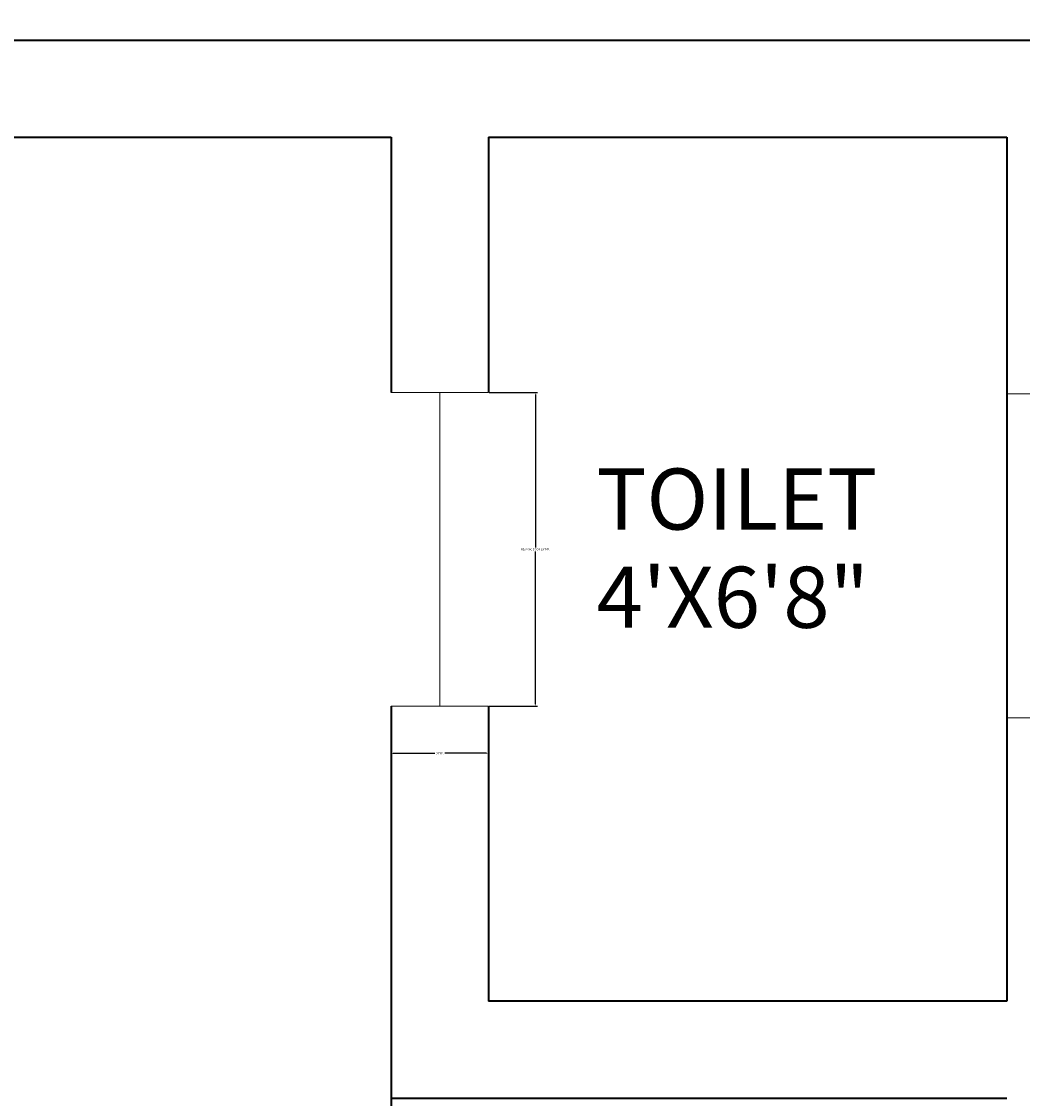
# Model space of a CAD drawing. Units: feet. Extents: x 2100 to 2836, y 2433 to 3396.
# Tile 9 of 12: x 2309 to 2402, y 3224 to 3324. Entities that reach past the tile are written whole.
import ezdxf

# ---------------------------------------------------------------- set-up
doc = ezdxf.new("R2010")
doc.units = ezdxf.units.FT
for name, color, linetype, lineweight in [('A-ANNO-DIMS', 2, 'Continuous', 18), ('A-AREA-IDEN', 7, 'Continuous', 18), ('A-DOOR', 3, 'Continuous', 18), ('A-GLAZ', 4, 'Continuous', 18), ('A-WALL', 7, 'Continuous', 35)]:
    doc.layers.add(name, color=color, linetype=linetype, lineweight=lineweight)
doc.styles.get("Standard").update_dxf_attribs({"font": 'arial.ttf'})
doc.dimstyles.get("Standard").update_dxf_attribs({"dimtxt": 0.18, "dimasz": 0.18, "dimexe": 0.18, "dimexo": 0.0625, "dimgap": 0.09, "dimtad": 0, "dimtih": 1, "dimtoh": 1, "dimdec": 4, "dimzin": 0, "dimdsep": 46, "dimtxsty": 'Standard', "dimcen": 0.09, "dimadec": 0, "dimazin": 0, "dimtfac": 1, "dimtdec": 4, "dimtofl": 0, "dimtmove": 0, "dimatfit": 3, "dimfxl": 1, "dimtolj": 1, "dimtzin": 0, "dimarcsym": 0})

# ---------------------------------------------------------------- blocks, each defined once
blk = doc.blocks.new('DOOR-REAR-TOILET')
for p, q in [((0, 29.05), (9, 29.05)), ((4.5, 29.05), (4.5, 0)), ((0, 0), (9, 0))]:
    blk.add_line(p, q)
blk = doc.blocks.new('*D30')
at = {"layer": 'A-ANNO-DIMS', "color": 0, "lineweight": -2, "transparency": 16777216}
for p, q in [((2352.748, 3289.173), (2357.223, 3289.173)), ((2357.043, 3288.993), (2357.043, 3274.831)), ((2357.043, 3260.303), (2357.043, 3274.465)), ((2352.748, 3260.123), (2357.223, 3260.123))]:
    blk.add_line(p, q, dxfattribs=at)
at = {"layer": 'A-ANNO-DIMS', "color": 0, "transparency": 16777216}
for points in [[(2357.013, 3288.993), (2357.073, 3288.993), (2357.043, 3289.173)], [(2357.013, 3260.303), (2357.073, 3260.303), (2357.043, 3260.123)]]:
    blk.add_solid(points, dxfattribs=at)
at = {"layer": 'Defpoints', "color": 0, "transparency": 16777216}
for p in [(2352.686, 3289.173), (2357.043, 3289.173), (2352.686, 3260.123)]:
    blk.add_point(p, dxfattribs=at)
at = {"layer": 'A-ANNO-DIMS', "color": 0, "transparency": 16777216, "insert": (2357.043, 3274.648), "char_height": 0.18, "attachment_point": 5}
blk.add_mtext('\\A1;REAR WC DOOR 29 TYP.', dxfattribs=at)
blk = doc.blocks.new('*D31')
at = {"layer": 'A-ANNO-DIMS', "color": 0, "lineweight": -2, "transparency": 16777216}
for p, q in [((2343.686, 3260.061), (2343.686, 3255.586)), ((2352.686, 3260.061), (2352.686, 3255.586)), ((2343.866, 3255.766), (2347.728, 3255.766)), ((2352.506, 3255.766), (2348.644, 3255.766))]:
    blk.add_line(p, q, dxfattribs=at)
at = {"layer": 'A-ANNO-DIMS', "color": 0, "transparency": 16777216}
for points in [[(2343.866, 3255.796), (2343.866, 3255.736), (2343.686, 3255.766)], [(2352.506, 3255.796), (2352.506, 3255.736), (2352.686, 3255.766)]]:
    blk.add_solid(points, dxfattribs=at)
at = {"layer": 'Defpoints', "color": 0, "transparency": 16777216}
for p in [(2343.686, 3260.123), (2352.686, 3260.123), (2352.686, 3255.766)]:
    blk.add_point(p, dxfattribs=at)
at = {"layer": 'A-ANNO-DIMS', "color": 0, "transparency": 16777216, "insert": (2348.186, 3255.766), "char_height": 0.18, "attachment_point": 5}
blk.add_mtext('\\A1;9 TYP.', dxfattribs=at)
blk = doc.blocks.new('*D40')
at = {"layer": 'A-ANNO-DIMS', "color": 0, "lineweight": -2, "transparency": 16777216}
for p, q in [((2190.686, 3321.866), (2190.686, 3396.054)), ((2190.866, 3395.874), (2299.895, 3395.874)), ((2409.506, 3395.874), (2300.476, 3395.874)), ((2409.686, 3321.866), (2409.686, 3396.054))]:
    blk.add_line(p, q, dxfattribs=at)
at = {"layer": 'A-ANNO-DIMS', "color": 0, "transparency": 16777216}
for points in [[(2190.866, 3395.904), (2190.866, 3395.844), (2190.686, 3395.874)], [(2409.506, 3395.904), (2409.506, 3395.844), (2409.686, 3395.874)]]:
    blk.add_solid(points, dxfattribs=at)
at = {"layer": 'Defpoints', "color": 0, "transparency": 16777216}
for p in [(2409.686, 3395.874), (2190.686, 3321.803), (2409.686, 3321.803)]:
    blk.add_point(p, dxfattribs=at)
at = {"layer": 'A-ANNO-DIMS', "color": 0, "transparency": 16777216, "insert": (2300.186, 3395.874), "char_height": 0.18, "attachment_point": 5}
blk.add_mtext('\\A1;219', dxfattribs=at)

msp = doc.modelspace()

# ---------------------------------------------------------------- linework, layer by layer
at = {"layer": 'A-GLAZ'}
for p, q in [((2400.6857, 3289.0453), (2409.6857, 3289.0453)), ((2400.6857, 3259.0368), (2409.6857, 3259.0368))]:
    msp.add_line(p, q, dxfattribs=at)
at = {"layer": 'A-WALL'}
for p, q in [((2190.6857, 3321.8031), (2343.6857, 3321.8031)), ((2190.6857, 3321.8031), (2409.6857, 3321.8031)), ((2199.6857, 3312.8031), (2343.6857, 3312.8031)), ((2343.6857, 3312.8031), (2343.6857, 3289.173)), ((2352.6857, 3312.8031), (2352.6857, 3289.173)), ((2352.6857, 3312.8031), (2400.6857, 3312.8031)), ((2400.6857, 3312.8031), (2400.6857, 3232.8031)), ((2343.6857, 3260.1235), (2343.6857, 3180.8031)), ((2352.6857, 3260.1235), (2352.6857, 3232.8031)), ((2400.6857, 3232.8031), (2352.6857, 3232.8031)), ((2400.6857, 3223.8031), (2343.6857, 3223.8031))]:
    msp.add_line(p, q, dxfattribs=at)

# ---------------------------------------------------------------- block references
at = {"layer": 'A-DOOR'}
msp.add_blockref('DOOR-REAR-TOILET', (2343.6857, 3260.1235), dxfattribs=at)

# ---------------------------------------------------------------- texts
at = {"layer": 'A-AREA-IDEN'}
for s, p in [('TOILET', (2362.6963, 3276.4772)), ('4\'X6\'8"', (2362.6963, 3267.3846))]:
    msp.add_text(s, height=5.66017, dxfattribs=at).set_placement(p)

# ---------------------------------------------------------------- dimensions: what is measured, and where the dimension line sits
at = {"layer": 'A-ANNO-DIMS'}
dim = msp.add_linear_dim(base=(2409.6857, 3395.8745), p1=(2190.6857, 3321.8031), p2=(2409.6857, 3321.8031), dimstyle='Standard', override={"dimdec": 0, "dimlfac": 1, "dimrnd": 0, "dimzin": 0, "dimdsep": 46, "dimlunit": 2}, dxfattribs=at)
dim.commit()
dim.dimension.update_dxf_attribs({"geometry": '*D40', "text_midpoint": (2300.1857, 3395.8745)})
dim = msp.add_linear_dim(base=(2357.0431, 3289.173), p1=(2352.6857, 3260.1235), p2=(2352.6857, 3289.173), angle=90, text='REAR WC DOOR <> TYP.', dimstyle='Standard', override={"dimdec": 0, "dimlfac": 1, "dimrnd": 0, "dimzin": 0, "dimdsep": 46, "dimlunit": 2}, dxfattribs=at)
dim.commit()
dim.dimension.update_dxf_attribs({"geometry": '*D30', "text_midpoint": (2357.0431, 3274.6482)})
dim = msp.add_linear_dim(base=(2352.6857, 3255.766), p1=(2343.6857, 3260.1235), p2=(2352.6857, 3260.1235), text='<> TYP.', dimstyle='Standard', override={"dimdec": 0, "dimlfac": 1, "dimrnd": 0, "dimzin": 0, "dimdsep": 46, "dimlunit": 2}, dxfattribs=at)
dim.commit()
dim.dimension.update_dxf_attribs({"geometry": '*D31', "text_midpoint": (2348.1857, 3255.766)})

doc.saveas('drawing.dxf')
